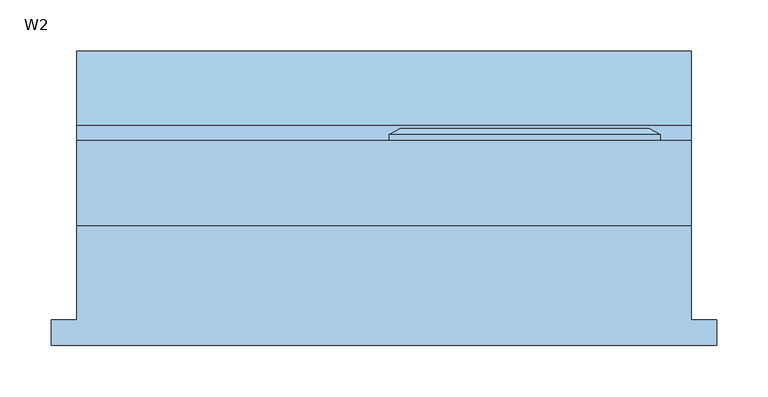
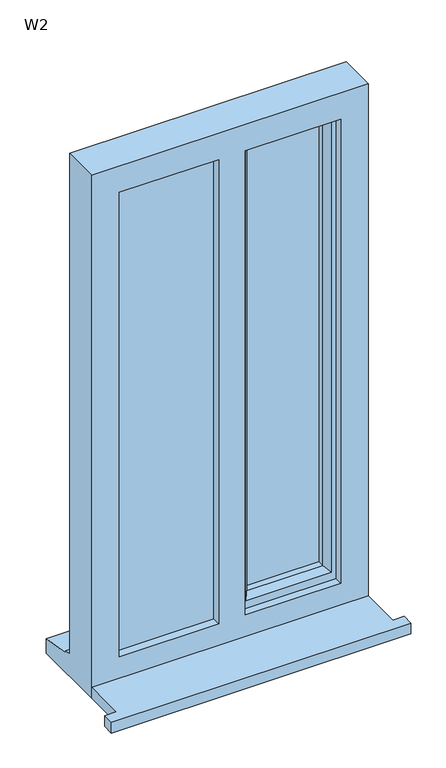
"""IFC4 building model written with IfcOpenShell, lengths in millimetres: window geometry, W2."""

from ifc_helpers import new_model, si_unit, frame, origin, place, context, project, spatial, polyline, outline, extrude, faceted_brep, source, transform, mapped, element, save


def w2_02e3e303(model_context):
    return source(origin(), model_context, "Body", "SolidModel", [
        extrude(outline(polyline([(-610.0, -129.0434322), (-610.0, -104.0434322), (-585.0, -104.0434322), (-585.0, -12.0434322), (15.0, -12.0434322), (15.0, -104.0434322), (40.0, -104.0434322), (40.0, -129.0434322), (-610.0, -129.0434322)])), frame((0.0, 0.0, 1200.0), z_axis=(0.0, 0.0, 1.0), x_axis=(1.0, 0.0, 0.0)), (0.0, 0.0, 1.0), 25.0),
        faceted_brep([(-280.0, 70.9565678, 2370.0), (-280.0, 76.7300705, 2370.0), (-280.0, 76.7300705, 1253.0), (-280.0, 70.9565678, 1253.0), (-270.0, 5.9565678, 2360.0), (-270.0, 70.9565678, 2360.0), (-270.0, 70.9565678, 1263.0), (-270.0, 5.9565678, 1263.0), (-230.0, 20.4494677, 2320.0), (-240.1480377, 5.9565678, 2330.1480377), (-240.1480377, 5.9565678, 1292.8519623), (-230.0, 20.4494677, 1303.0), (-230.0, 34.9565678, 2320.0), (-230.0, 34.9565678, 1303.0), (-240.0, 58.9565678, 2330.0), (-240.0, 34.9565678, 2330.0), (-240.0, 34.9565678, 1293.0), (-240.0, 58.9565678, 1293.0), (-230.0, 76.7300705, 2320.0), (-230.0, 58.9565678, 2320.0), (-230.0, 58.9565678, 1303.0), (-230.0, 76.7300705, 1303.0), (-247.4457548, 82.5035732, 2337.4457548), (-247.4457548, 82.5035732, 1285.5542452), (-269.2153903, 82.5035732, 2359.2153903), (-269.2153903, 82.5035732, 1263.7846097), (-15.0, 76.7300705, 1253.0), (-15.0, 70.9565678, 1253.0), (-25.0, 70.9565678, 1263.0), (-25.0, 5.9565678, 1263.0), (-54.8519623, 5.9565678, 1292.8519623), (-65.0, 20.4494677, 1303.0), (-65.0, 34.9565678, 1303.0), (-55.0, 34.9565678, 1293.0), (-55.0, 58.9565678, 1293.0), (-65.0, 58.9565678, 1303.0), (-65.0, 76.7300705, 1303.0), (-47.5542452, 82.5035732, 1285.5542452), (-25.7846097, 82.5035732, 1263.7846097), (-15.0, 76.7300705, 2370.0), (-15.0, 70.9565678, 2370.0), (-25.0, 70.9565678, 2360.0), (-25.0, 5.9565678, 2360.0), (-54.8519623, 5.9565678, 2330.1480377), (-65.0, 20.4494677, 2320.0), (-65.0, 34.9565678, 2320.0), (-55.0, 34.9565678, 2330.0), (-55.0, 58.9565678, 2330.0), (-65.0, 58.9565678, 2320.0), (-65.0, 76.7300705, 2320.0), (-47.5542452, 82.5035732, 2337.4457548), (-25.7846097, 82.5035732, 2359.2153903)], [[[0, 1, 2, 3]], [[4, 5, 6, 7]], [[8, 9, 10, 11]], [[12, 8, 11, 13]], [[14, 15, 16, 17]], [[18, 19, 20, 21]], [[22, 18, 21, 23]], [[1, 24, 25, 2]], [[3, 2, 26, 27]], [[7, 6, 28, 29]], [[11, 10, 30, 31]], [[13, 11, 31, 32]], [[17, 16, 33, 34]], [[21, 20, 35, 36]], [[23, 21, 36, 37]], [[2, 25, 38, 26]], [[27, 26, 39, 40]], [[29, 28, 41, 42]], [[31, 30, 43, 44]], [[32, 31, 44, 45]], [[34, 33, 46, 47]], [[36, 35, 48, 49]], [[37, 36, 49, 50]], [[26, 38, 51, 39]], [[40, 39, 1, 0]], [[3, 27, 40, 0], [5, 41, 28, 6]], [[42, 41, 5, 4]], [[7, 29, 42, 4], [9, 43, 30, 10]], [[44, 43, 9, 8]], [[45, 44, 8, 12]], [[15, 46, 33, 16], [13, 32, 45, 12]], [[47, 46, 15, 14]], [[17, 34, 47, 14], [19, 48, 35, 20]], [[49, 48, 19, 18]], [[50, 49, 18, 22]], [[24, 51, 38, 25], [23, 37, 50, 22]], [[39, 51, 24, 1]]]),
        extrude(outline(polyline([(2340.0, -310.0), (2360.0, -310.0), (2360.0, -545.0), (1263.0, -545.0), (1263.0, -310.0), (1283.0, -310.0), (1283.0, -525.0), (2340.0, -525.0), (2340.0, -310.0)])), frame((0.0, 29.9565678, 0.0), z_axis=(0.0, 1.0, 0.0), x_axis=(0.0, 0.0, 1.0)), (0.0, 0.0, 1.0), 41.0),
        faceted_brep([(15.0, -12.0434322, 2400.0), (-585.0, -12.0434322, 2400.0), (-585.0, -12.0434322, 1200.0), (15.0, -12.0434322, 1200.0), (-45.0, -12.0434322, 2340.0), (-45.0, -12.0434322, 1275.0), (-252.0, -12.0434322, 1275.0), (-252.0, -12.0434322, 2340.0), (-310.0, -12.0434322, 2340.0), (-310.0, -12.0434322, 1275.0), (-525.0, -12.0434322, 1275.0), (-525.0, -12.0434322, 2340.0), (-585.0, 70.9565678, 2400.0), (-585.0, 70.9565678, 1251.0), (-585.0, 85.9565678, 1249.68767), (-585.0, 85.9565678, 1244.7449676), (-585.0, 158.4565678, 1233.8088847), (-585.0, 158.4565678, 1200.0), (15.0, 70.9565678, 2400.0), (15.0, 70.9565678, 1251.0), (-545.0, 70.9565678, 2360.0), (-545.0, 70.9565678, 1263.0), (-310.0, 70.9565678, 1263.0), (-310.0, 70.9565678, 2360.0), (-270.0, 70.9565678, 2360.0), (-270.0, 70.9565678, 1263.0), (-25.0, 70.9565678, 1263.0), (-25.0, 70.9565678, 2360.0), (-545.0, 5.9565678, 2360.0), (-545.0, 5.9565678, 1263.0), (-300.0, 5.9565678, 2360.0), (-300.0, 5.9565678, 1263.0), (-310.0, 5.9565678, 2340.0), (-525.0, 5.9565678, 2340.0), (-525.0, 5.9565678, 1275.0), (-310.0, 5.9565678, 1275.0), (-270.0, 5.9565678, 2360.0), (-25.0, 5.9565678, 2360.0), (-25.0, 5.9565678, 1263.0), (-270.0, 5.9565678, 1263.0), (-45.0, 5.9565678, 2340.0), (-252.0, 5.9565678, 2340.0), (-252.0, 5.9565678, 1275.0), (-45.0, 5.9565678, 1275.0), (-310.0, 29.9565678, 2360.0), (-300.0, 29.9565678, 2360.0), (15.0, 158.4565678, 1200.0), (15.0, 158.4565678, 1233.8088847), (15.0, 85.9565678, 1244.7449676), (15.0, 85.9565678, 1249.68767), (-300.0, 29.9565678, 1263.0), (-310.0, 29.9565678, 1263.0)], [[[0, 1, 2, 3], [4, 5, 6, 7], [8, 9, 10, 11]], [[2, 1, 12, 13, 14, 15, 16, 17]], [[13, 12, 18, 19], [20, 21, 22, 23], [24, 25, 26, 27]], [[21, 20, 28, 29]], [[28, 30, 31, 29], [32, 33, 34, 35]], [[36, 37, 38, 39], [40, 41, 42, 43]], [[33, 11, 10, 34]], [[1, 0, 18, 12]], [[28, 20, 23, 44, 45, 30]], [[27, 37, 36, 24]], [[11, 33, 32, 8]], [[40, 4, 7, 41]], [[19, 18, 0, 3, 46, 47, 48, 49]], [[27, 26, 38, 37]], [[4, 40, 43, 5]], [[45, 50, 31, 30]], [[50, 45, 44, 51]], [[51, 44, 23, 22]], [[25, 24, 36, 39]], [[41, 7, 6, 42]], [[8, 32, 35, 9]], [[46, 3, 2, 17]], [[47, 46, 17, 16]], [[48, 47, 16, 15]], [[49, 48, 15, 14]], [[19, 49, 14, 13]], [[22, 21, 29, 31, 50, 51]], [[26, 25, 39, 38]], [[6, 5, 43, 42]], [[35, 34, 10, 9]]]),
        extrude(outline(polyline([(-545.0, 29.9565678), (-300.0, 29.9565678), (-300.0, 5.9565678), (-545.0, 5.9565678), (-545.0, 29.9565678)])), frame((0.0, 0.0, 1263.0), z_axis=(0.0, 0.0, 1.0), x_axis=(1.0, 0.0, 0.0)), (0.0, 0.0, 1.0), 1097.0),
        extrude(outline(polyline([(-55.0, 34.9565678), (-240.0, 34.9565678), (-240.0, 58.9565678), (-55.0, 58.9565678), (-55.0, 34.9565678)])), frame((0.0, 0.0, 1293.0), z_axis=(0.0, 0.0, 1.0), x_axis=(1.0, 0.0, 0.0)), (0.0, 0.0, 1.0), 1037.0),
    ])


if __name__ == "__main__":
    model = new_model("IFC4")
    model_context = context("Model", 3, world=origin())
    ifc_project = project(units=[si_unit("LENGTHUNIT", "METRE", prefix="MILLI")], contexts=[model_context])
    site = spatial("IfcSite", under=ifc_project)
    building = spatial("IfcBuilding", under=site)
    placement = place(None, origin())
    w2_shape = w2_02e3e303(model_context)
    element("IfcWindow", 1, ObjectType="W2", at=placement, inside=building, context=model_context, shape_type="MappedRepresentation", body=[
        mapped(w2_shape, transform((0.0, 0.0, 0.0), x_axis=(1.0, 0.0, 0.0), y_axis=(0.0, 1.0, 0.0), z_axis=(0.0, 0.0, 1.0))),
    ])
    save(model, "model.ifc")

# Revit data of these elements
# Type "W2"
#   Type Mark = "42"
#   Operation = "DoublePanelVertical"
#   Manufacturer = "Revit"
#   Wrap Layers (Ext) from Ext = 102.5 mm
#   Wrap Layers (Int) from Ext = 177.5 mm
#   Window Board Projection = 25 mm
#   Window Board Extension = 25 mm
#   Rough Width = 600 mm
#   Rough Height = 1200 mm
#   Height = 1200 mm
#   Width = 600 mm
#   Glazing Thickness = 24 mm
#   FrameOffset - External = 50 mm
#   Frame Depth = 65 mm
#   Default Head Height = 2400 mm
#   Cill Depth = 87.5 mm
#   Cavity Closer Width = 50 mm
#   Cavity Closer Offset from Ext = 102.5 mm
#   Cavity Closer Depth = 85 mm
#   Vis - Cavity Closers = yes
#   Material Trim = Window Frame
#   Material Glass = Glass
#   Material Frame = Window Frame
#   Wall Closure = (empty or 0)
# Element 1 (IfcWindow, "W2")
#   Materials on its faces: "Window Frame", "Glass"
# Materials
#   "Window Frame": colour RGB 249 249 249, transparency 0
#   "Glass": class "Glass", colour RGB 245 245 243, transparency 1, Description = "Soda Lime Glass", Cost = 0
